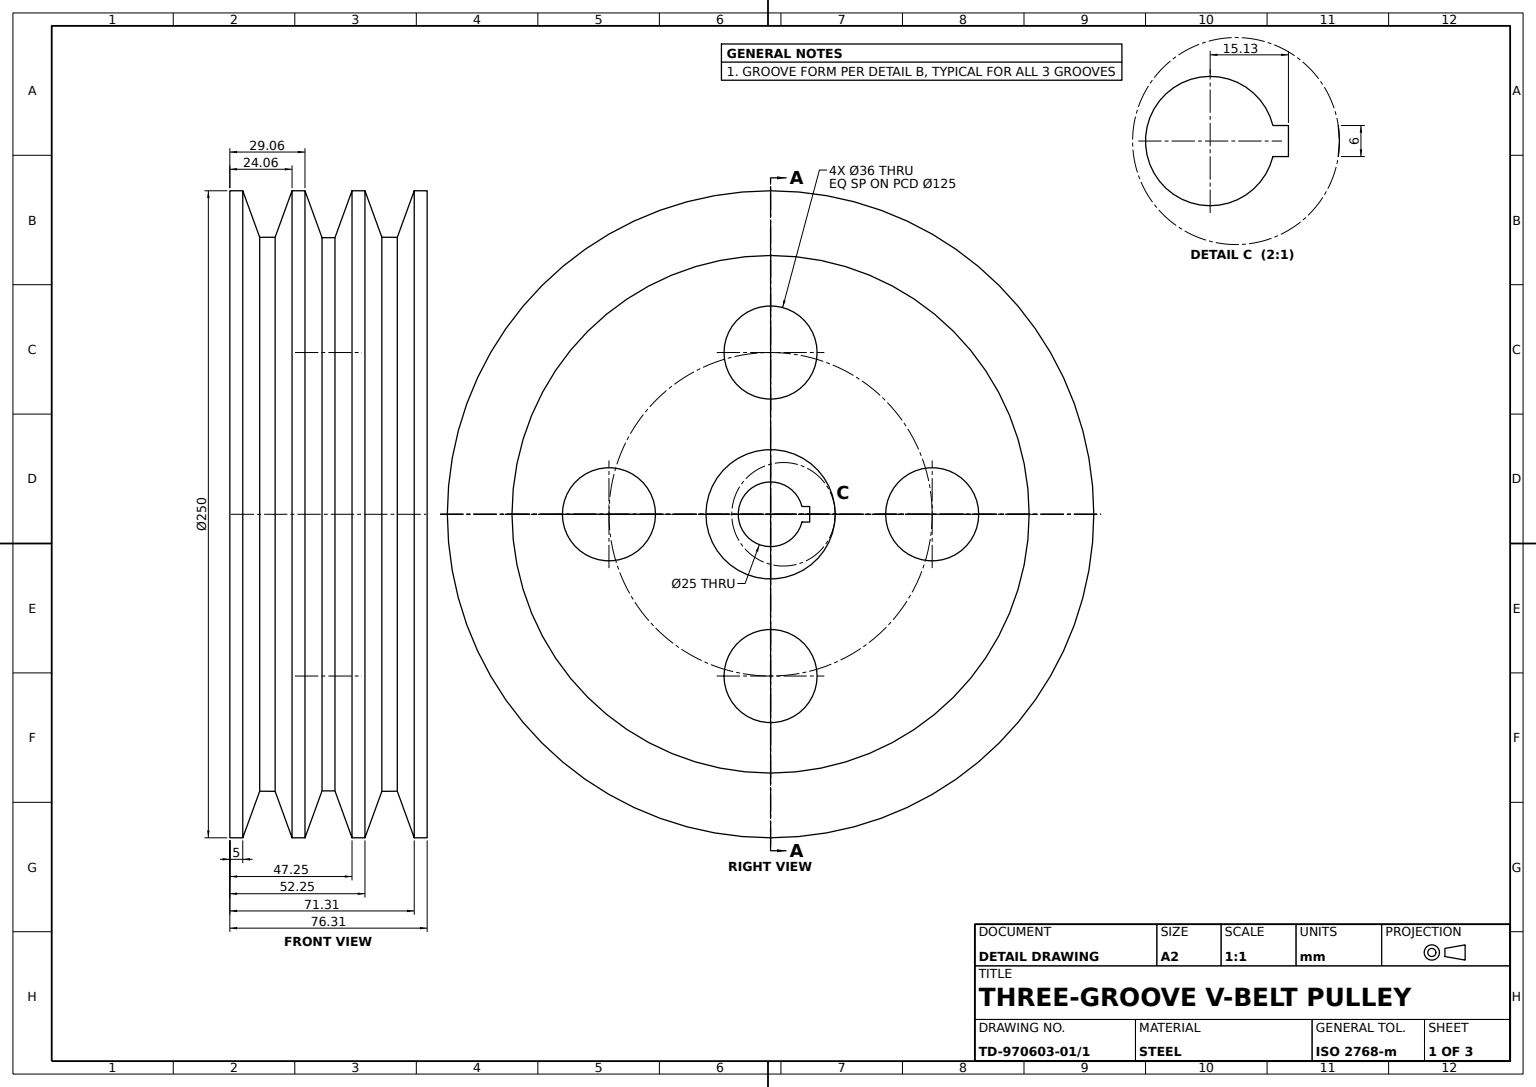
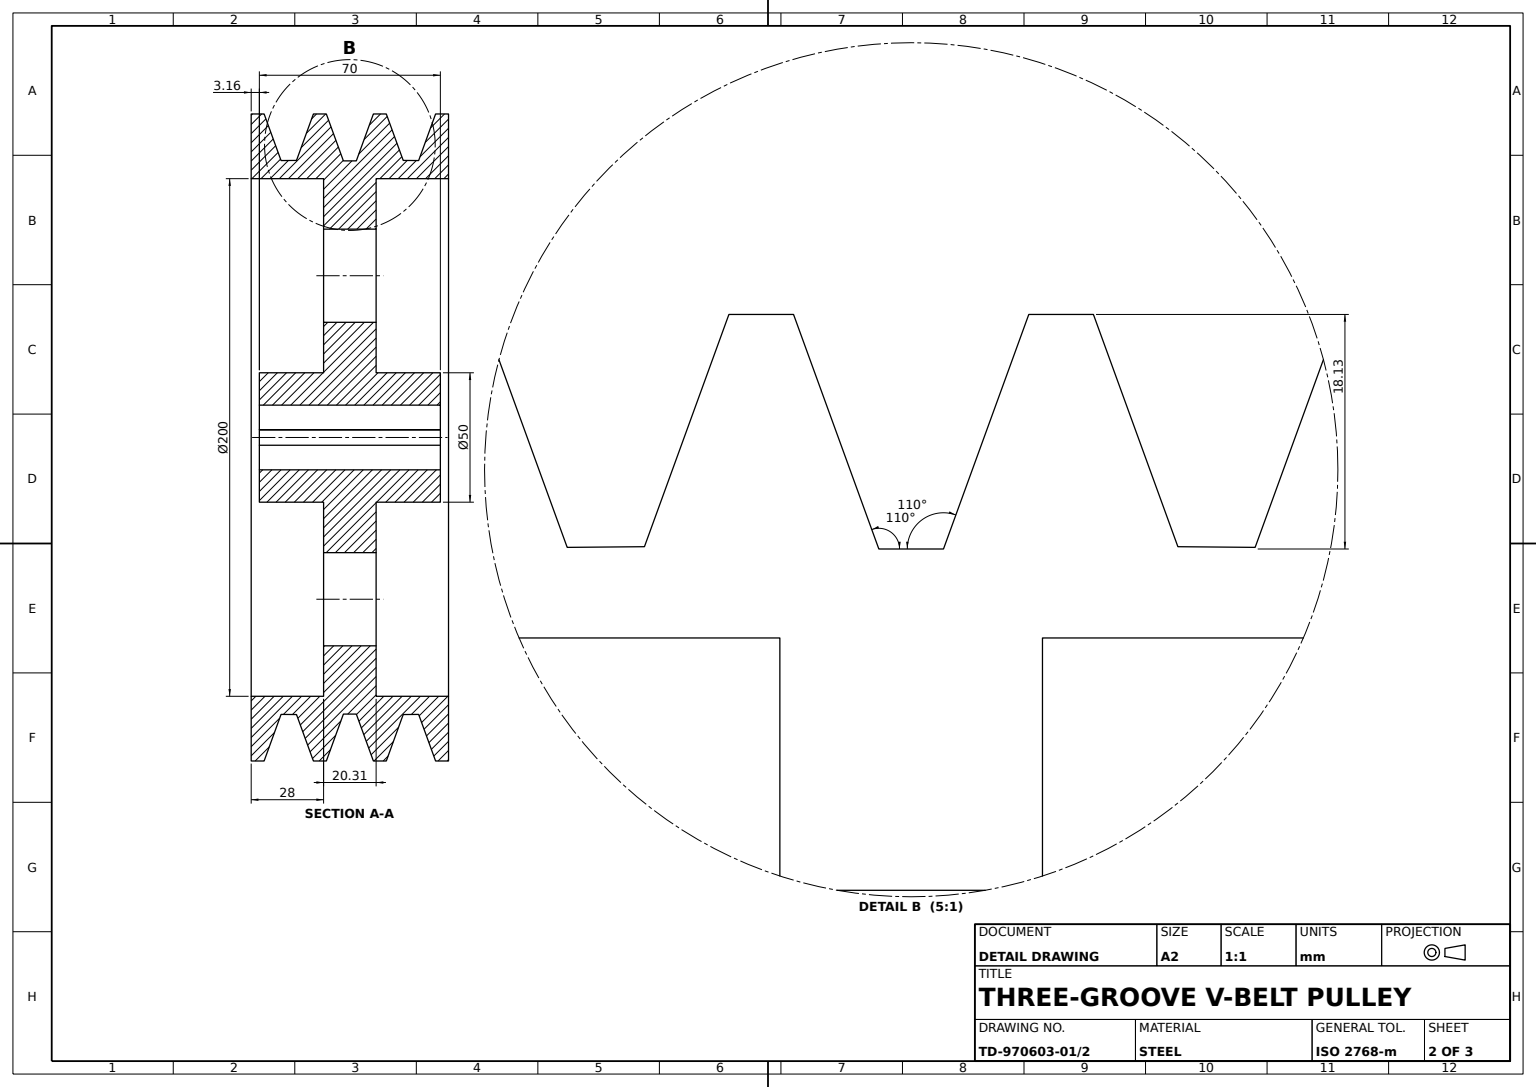
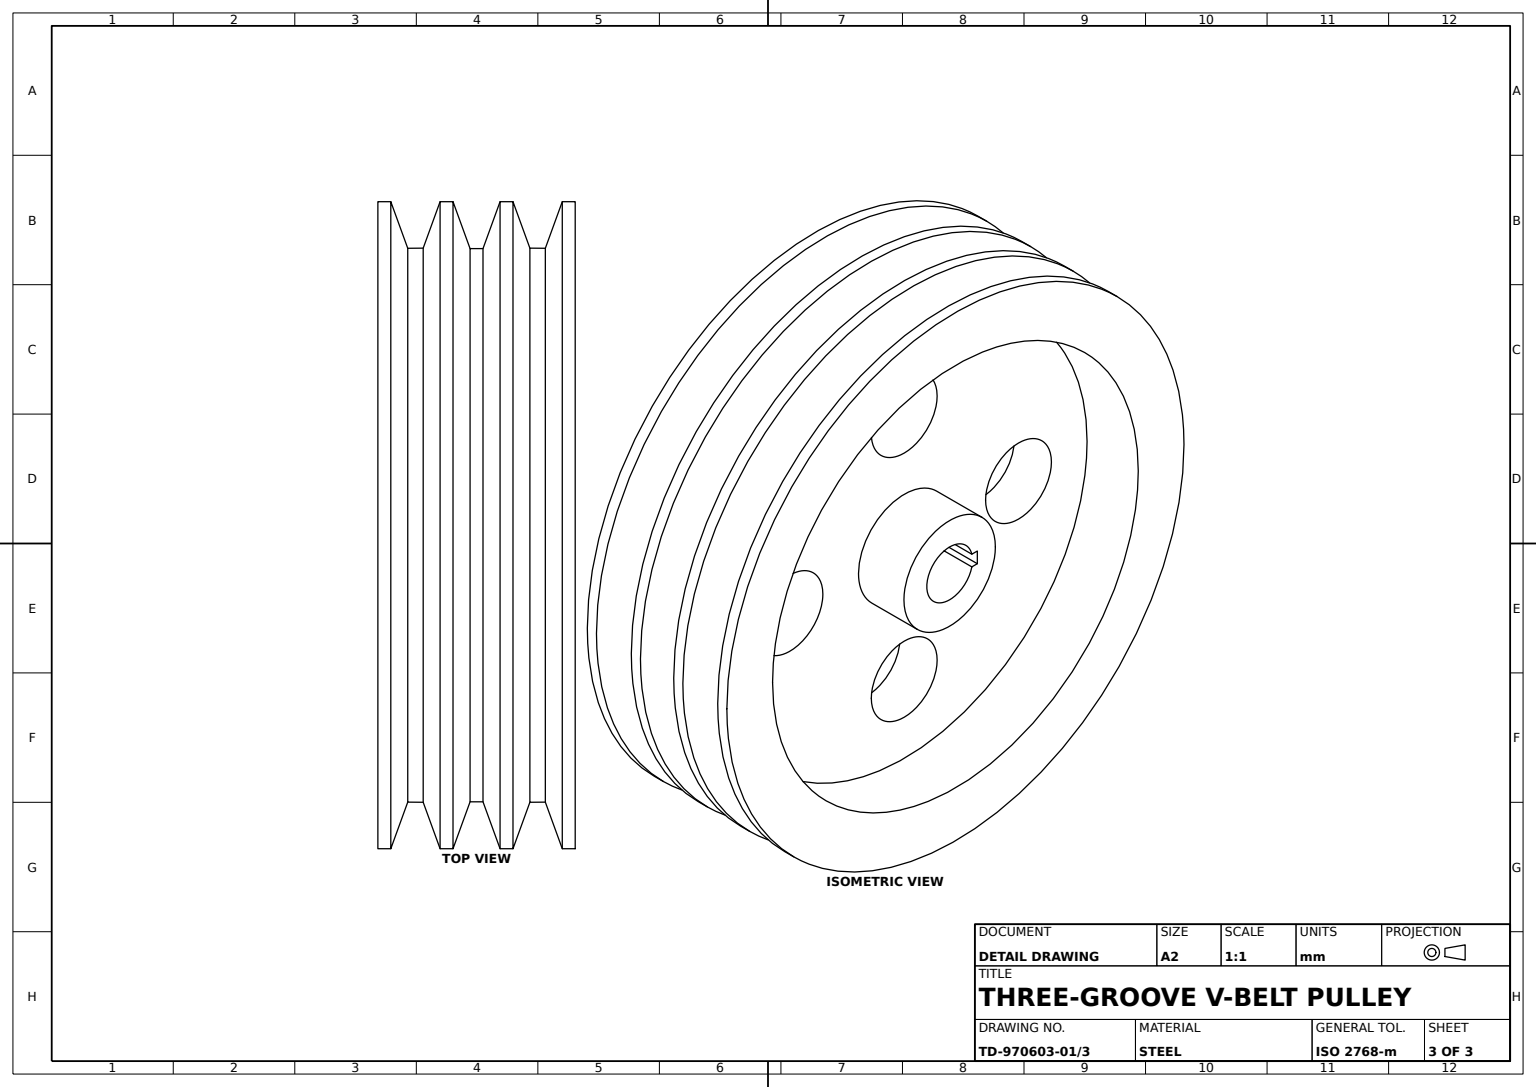
from build123d import *

# Parameters (mm, degrees)
WEB_RECESS_SKETCH_R       = 100
WEB_RECESS_200_DEPTH      = 28
LIGHTENING_HOLES_SKETCH_R = 18
LIGHTENING_HOLES_4X_DEPTH = 11
HUB_SKETCH_R              = 25
HUB_50_DEPTH              = 35
BORE_SKETCH_R             = 12.5
BORE_25_DEPTH             = 35
KEYWAY_SKETCH_W           = 3
KEYWAY_SKETCH_H           = 6
KEYWAY_6X3_DEPTH          = 35


with BuildPart() as part:
    # Pulley Profile Sketch → Pulley Body 3-Groove (revolve)
    with BuildSketch(Plane.XY, mode=Mode.PRIVATE) as pulley_body_3_groove_sk:
        Polygon((-38.155633051, 12.5), (38.155633051, 12.5), (38.155633051, 125), (33.155633051, 125), (26.604168834, 107), (20.629224678, 107.05281598), (14.096983906, 125), (9.096983906, 125), (2.5, 106.874935681), (-2.5, 106.874935681), (-9.096983906, 125), (-14.096983906, 125), (-20.629224678, 107.05281598), (-26.604168834, 107), (-33.155633051, 125), (-38.155633051, 125), align=None)
    revolve(pulley_body_3_groove_sk.sketch.rotate(Axis((-177.514342584, 0, 0), (1, 0, 0)), 90), axis=Axis((-177.514342584, 0, 0), (1, 0, 0)))

    # Web Recess Sketch → Web Recess Ø200 (cut)
    with BuildSketch(Plane(origin=(38.155633051, 0, 0), x_dir=(0, 0, -1), z_dir=(1, 0, 0))):
        Circle(WEB_RECESS_SKETCH_R)
    web_recess_200 = extrude(amount=-WEB_RECESS_200_DEPTH, mode=Mode.SUBTRACT)

    # Web Recess Mirror: Web Recess Ø200 across plane
    add(web_recess_200.mirror(Plane(origin=(0, 0, 0), x_dir=(0, 0, 1), z_dir=(1, 0, 0))), mode=Mode.SUBTRACT)

    # Lightening Holes Sketch → Lightening Holes 4x (cut, symmetric)
    with BuildSketch(Plane(origin=(0, 0, 0), x_dir=(0, 0, -1), z_dir=(1, 0, 0))):
        with Locations((0, 62.5)):
            Circle(LIGHTENING_HOLES_SKETCH_R)
        with Locations((62.5, 0)):
            Circle(LIGHTENING_HOLES_SKETCH_R)
        with Locations((0, -62.5)):
            Circle(LIGHTENING_HOLES_SKETCH_R)
        with Locations((-62.5, 0)):
            Circle(LIGHTENING_HOLES_SKETCH_R)
    extrude(amount=LIGHTENING_HOLES_4X_DEPTH, both=True, mode=Mode.SUBTRACT)

    # Hub Sketch → Hub Ø50 (add, symmetric)
    with BuildSketch(Plane(origin=(0, 0, 0), x_dir=(0, 0, -1), z_dir=(1, 0, 0))):
        with Locations(Location((0, 0, 0), (0, 0, 180))):
            Circle(HUB_SKETCH_R)
    extrude(amount=HUB_50_DEPTH, both=True)

    # Bore Sketch → Bore Ø25 (cut, symmetric)
    with BuildSketch(Plane(origin=(0, 0, 0), x_dir=(0, 0, -1), z_dir=(1, 0, 0))):
        Circle(BORE_SKETCH_R)
    extrude(amount=BORE_25_DEPTH, both=True, mode=Mode.SUBTRACT)

    # Keyway Sketch → Keyway 6x3 (cut, symmetric)
    with BuildSketch(Plane(origin=(0, 0, 0), x_dir=(0, 0, -1), z_dir=(1, 0, 0))):
        with Locations((13.6346611, 0)):
            Rectangle(KEYWAY_SKETCH_W, KEYWAY_SKETCH_H)
    extrude(amount=KEYWAY_6X3_DEPTH, both=True, mode=Mode.SUBTRACT)


solid = part.part
